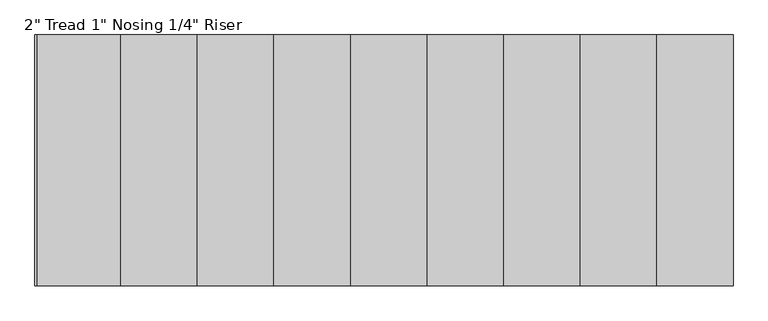
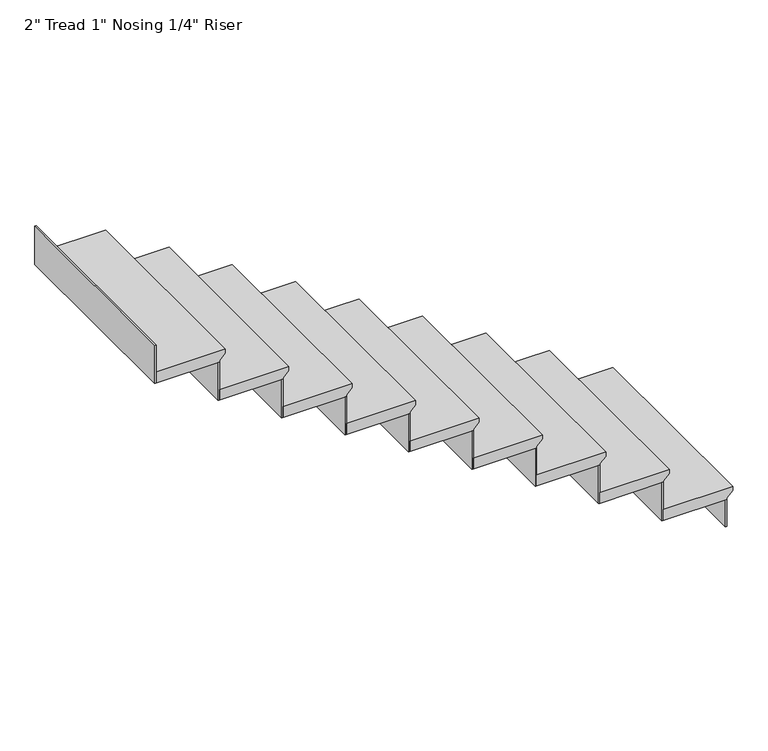
"""IFC4 building model written with IfcOpenShell, lengths in millimetres: stair flight geometry."""

from ifc_helpers import new_model, si_unit, origin, place, context, project, spatial, faceted_brep, source, transform, mapped, element, save


def stair_flight_6bca3b3f(model_context):
    return source(origin(), model_context, "Body", "Brep", [
        faceted_brep([(-9543.8120641, -2647.9669819, 3968.75), (-9543.8120641, -2647.9669819, 3987.8), (-9543.8120641, -3562.3669819, 3987.8), (-9543.8120641, -3562.3669819, 3968.75), (-9569.2120641, -2647.9669819, 3943.35), (-9569.2120641, -3562.3669819, 3943.35), (-9848.6120641, -2647.9669819, 3987.8), (-9848.6120641, -3562.3669819, 3987.8), (-9569.2120641, -3562.3669819, 3937.0), (-9848.6120641, -3562.3669819, 3937.0), (-9848.6120641, -2647.9669819, 3937.0), (-9569.2120641, -2647.9669819, 3937.0)], [[[0, 1, 2, 3]], [[4, 0, 3, 5]], [[2, 1, 6, 7]], [[8, 9, 10, 11]], [[2, 7, 9, 8, 5, 3]], [[8, 11, 4, 5]], [[6, 1, 0, 4, 11, 10]], [[7, 6, 10, 9]]]),
        faceted_brep([(-9569.2120641, -2647.9669819, 3937.0), (-9569.2120641, -2647.9669819, 3810.0), (-9575.5620641, -2647.9669819, 3810.0), (-9575.5620641, -2647.9669819, 3937.0), (-9569.2120641, -3562.3669819, 3937.0), (-9575.5620641, -3562.3669819, 3937.0), (-9575.5620641, -3562.3669819, 3810.0), (-9569.2120641, -3562.3669819, 3810.0)], [[[0, 1, 2, 3]], [[4, 5, 6, 7]], [[1, 0, 4, 7]], [[2, 1, 7, 6]], [[3, 2, 6, 5]], [[0, 3, 5, 4]]]),
        faceted_brep([(-9848.6120641, -2647.9669819, 4114.8), (-9848.6120641, -2647.9669819, 3937.0), (-9854.9620641, -2647.9669819, 3937.0), (-9854.9620641, -2647.9669819, 4114.8), (-9848.6120641, -3562.3669819, 4114.8), (-9854.9620641, -3562.3669819, 4114.8), (-9854.9620641, -3562.3669819, 3937.0), (-9848.6120641, -3562.3669819, 3937.0)], [[[0, 1, 2, 3]], [[4, 5, 6, 7]], [[1, 0, 4, 7]], [[2, 1, 7, 6]], [[3, 2, 6, 5]], [[0, 3, 5, 4]]]),
        faceted_brep([(-9823.2120641, -3562.3669819, 4165.6), (-9823.2120641, -2647.9669819, 4165.6), (-10128.0120641, -2647.9669819, 4165.6), (-10128.0120641, -3562.3669819, 4165.6), (-9848.6120641, -3562.3669819, 4114.8), (-10128.0120641, -3562.3669819, 4114.8), (-10128.0120641, -2647.9669819, 4114.8), (-9848.6120641, -2647.9669819, 4114.8), (-9848.6120641, -3562.3669819, 4121.15), (-9823.2120641, -3562.3669819, 4146.55), (-9848.6120641, -2647.9669819, 4121.15), (-9823.2120641, -2647.9669819, 4146.55)], [[[0, 1, 2, 3]], [[4, 5, 6, 7]], [[0, 3, 5, 4, 8, 9]], [[4, 7, 10, 8]], [[2, 1, 11, 10, 7, 6]], [[3, 2, 6, 5]], [[11, 1, 0, 9]], [[10, 11, 9, 8]]]),
        faceted_brep([(-10128.0120641, -2647.9669819, 4292.6), (-10128.0120641, -2647.9669819, 4114.8), (-10134.3620641, -2647.9669819, 4114.8), (-10134.3620641, -2647.9669819, 4292.6), (-10128.0120641, -3562.3669819, 4292.6), (-10134.3620641, -3562.3669819, 4292.6), (-10134.3620641, -3562.3669819, 4114.8), (-10128.0120641, -3562.3669819, 4114.8)], [[[0, 1, 2, 3]], [[4, 5, 6, 7]], [[1, 0, 4, 7]], [[2, 1, 7, 6]], [[3, 2, 6, 5]], [[0, 3, 5, 4]]]),
        faceted_brep([(-10102.6120641, -3562.3669819, 4343.4), (-10102.6120641, -2647.9669819, 4343.4), (-10407.4120641, -2647.9669819, 4343.4), (-10407.4120641, -3562.3669819, 4343.4), (-10128.0120641, -3562.3669819, 4292.6), (-10407.4120641, -3562.3669819, 4292.6), (-10407.4120641, -2647.9669819, 4292.6), (-10128.0120641, -2647.9669819, 4292.6), (-10128.0120641, -3562.3669819, 4298.95), (-10102.6120641, -3562.3669819, 4324.35), (-10128.0120641, -2647.9669819, 4298.95), (-10102.6120641, -2647.9669819, 4324.35)], [[[0, 1, 2, 3]], [[4, 5, 6, 7]], [[0, 3, 5, 4, 8, 9]], [[4, 7, 10, 8]], [[2, 1, 11, 10, 7, 6]], [[3, 2, 6, 5]], [[11, 1, 0, 9]], [[10, 11, 9, 8]]]),
        faceted_brep([(-10407.4120641, -2647.9669819, 4470.4), (-10407.4120641, -2647.9669819, 4292.6), (-10413.7620641, -2647.9669819, 4292.6), (-10413.7620641, -2647.9669819, 4470.4), (-10407.4120641, -3562.3669819, 4470.4), (-10413.7620641, -3562.3669819, 4470.4), (-10413.7620641, -3562.3669819, 4292.6), (-10407.4120641, -3562.3669819, 4292.6)], [[[0, 1, 2, 3]], [[4, 5, 6, 7]], [[1, 0, 4, 7]], [[2, 1, 7, 6]], [[3, 2, 6, 5]], [[0, 3, 5, 4]]]),
        faceted_brep([(-10382.0120641, -3562.3669819, 4521.2), (-10382.0120641, -2647.9669819, 4521.2), (-10686.8120641, -2647.9669819, 4521.2), (-10686.8120641, -3562.3669819, 4521.2), (-10407.4120641, -3562.3669819, 4470.4), (-10686.8120641, -3562.3669819, 4470.4), (-10686.8120641, -2647.9669819, 4470.4), (-10407.4120641, -2647.9669819, 4470.4), (-10407.4120641, -3562.3669819, 4476.75), (-10382.0120641, -3562.3669819, 4502.15), (-10407.4120641, -2647.9669819, 4476.75), (-10382.0120641, -2647.9669819, 4502.15)], [[[0, 1, 2, 3]], [[4, 5, 6, 7]], [[0, 3, 5, 4, 8, 9]], [[4, 7, 10, 8]], [[2, 1, 11, 10, 7, 6]], [[3, 2, 6, 5]], [[11, 1, 0, 9]], [[10, 11, 9, 8]]]),
        faceted_brep([(-10686.8120641, -2647.9669819, 4648.2), (-10686.8120641, -2647.9669819, 4470.4), (-10693.1620641, -2647.9669819, 4470.4), (-10693.1620641, -2647.9669819, 4648.2), (-10686.8120641, -3562.3669819, 4648.2), (-10693.1620641, -3562.3669819, 4648.2), (-10693.1620641, -3562.3669819, 4470.4), (-10686.8120641, -3562.3669819, 4470.4)], [[[0, 1, 2, 3]], [[4, 5, 6, 7]], [[1, 0, 4, 7]], [[2, 1, 7, 6]], [[3, 2, 6, 5]], [[0, 3, 5, 4]]]),
        faceted_brep([(-10661.4120641, -3562.3669819, 4699.0), (-10661.4120641, -2647.9669819, 4699.0), (-10966.2120641, -2647.9669819, 4699.0), (-10966.2120641, -3562.3669819, 4699.0), (-10686.8120641, -3562.3669819, 4648.2), (-10966.2120641, -3562.3669819, 4648.2), (-10966.2120641, -2647.9669819, 4648.2), (-10686.8120641, -2647.9669819, 4648.2), (-10686.8120641, -3562.3669819, 4654.55), (-10661.4120641, -3562.3669819, 4679.95), (-10686.8120641, -2647.9669819, 4654.55), (-10661.4120641, -2647.9669819, 4679.95)], [[[0, 1, 2, 3]], [[4, 5, 6, 7]], [[0, 3, 5, 4, 8, 9]], [[4, 7, 10, 8]], [[2, 1, 11, 10, 7, 6]], [[3, 2, 6, 5]], [[11, 1, 0, 9]], [[10, 11, 9, 8]]]),
        faceted_brep([(-10966.2120641, -2647.9669819, 4826.0), (-10966.2120641, -2647.9669819, 4648.2), (-10972.5620641, -2647.9669819, 4648.2), (-10972.5620641, -2647.9669819, 4826.0), (-10966.2120641, -3562.3669819, 4826.0), (-10972.5620641, -3562.3669819, 4826.0), (-10972.5620641, -3562.3669819, 4648.2), (-10966.2120641, -3562.3669819, 4648.2)], [[[0, 1, 2, 3]], [[4, 5, 6, 7]], [[1, 0, 4, 7]], [[2, 1, 7, 6]], [[3, 2, 6, 5]], [[0, 3, 5, 4]]]),
        faceted_brep([(-10940.8120641, -3562.3669819, 4876.8), (-10940.8120641, -2647.9669819, 4876.8), (-11245.6120641, -2647.9669819, 4876.8), (-11245.6120641, -3562.3669819, 4876.8), (-10966.2120641, -3562.3669819, 4826.0), (-11245.6120641, -3562.3669819, 4826.0), (-11245.6120641, -2647.9669819, 4826.0), (-10966.2120641, -2647.9669819, 4826.0), (-10966.2120641, -3562.3669819, 4832.35), (-10940.8120641, -3562.3669819, 4857.75), (-10966.2120641, -2647.9669819, 4832.35), (-10940.8120641, -2647.9669819, 4857.75)], [[[0, 1, 2, 3]], [[4, 5, 6, 7]], [[0, 3, 5, 4, 8, 9]], [[4, 7, 10, 8]], [[2, 1, 11, 10, 7, 6]], [[3, 2, 6, 5]], [[11, 1, 0, 9]], [[10, 11, 9, 8]]]),
        faceted_brep([(-11245.6120641, -2647.9669819, 5003.8), (-11245.6120641, -2647.9669819, 4826.0), (-11251.9620641, -2647.9669819, 4826.0), (-11251.9620641, -2647.9669819, 5003.8), (-11245.6120641, -3562.3669819, 5003.8), (-11251.9620641, -3562.3669819, 5003.8), (-11251.9620641, -3562.3669819, 4826.0), (-11245.6120641, -3562.3669819, 4826.0)], [[[0, 1, 2, 3]], [[4, 5, 6, 7]], [[1, 0, 4, 7]], [[2, 1, 7, 6]], [[3, 2, 6, 5]], [[0, 3, 5, 4]]]),
        faceted_brep([(-11220.2120641, -3562.3669819, 5054.6), (-11220.2120641, -2647.9669819, 5054.6), (-11525.0120641, -2647.9669819, 5054.6), (-11525.0120641, -3562.3669819, 5054.6), (-11245.6120641, -3562.3669819, 5003.8), (-11525.0120641, -3562.3669819, 5003.8), (-11525.0120641, -2647.9669819, 5003.8), (-11245.6120641, -2647.9669819, 5003.8), (-11245.6120641, -3562.3669819, 5010.15), (-11220.2120641, -3562.3669819, 5035.55), (-11245.6120641, -2647.9669819, 5010.15), (-11220.2120641, -2647.9669819, 5035.55)], [[[0, 1, 2, 3]], [[4, 5, 6, 7]], [[0, 3, 5, 4, 8, 9]], [[4, 7, 10, 8]], [[2, 1, 11, 10, 7, 6]], [[3, 2, 6, 5]], [[11, 1, 0, 9]], [[10, 11, 9, 8]]]),
        faceted_brep([(-11525.0120641, -2647.9669819, 5181.6), (-11525.0120641, -2647.9669819, 5003.8), (-11531.3620641, -2647.9669819, 5003.8), (-11531.3620641, -2647.9669819, 5181.6), (-11525.0120641, -3562.3669819, 5181.6), (-11531.3620641, -3562.3669819, 5181.6), (-11531.3620641, -3562.3669819, 5003.8), (-11525.0120641, -3562.3669819, 5003.8)], [[[0, 1, 2, 3]], [[4, 5, 6, 7]], [[1, 0, 4, 7]], [[2, 1, 7, 6]], [[3, 2, 6, 5]], [[0, 3, 5, 4]]]),
        faceted_brep([(-11499.6120641, -3562.3669819, 5232.4), (-11499.6120641, -2647.9669819, 5232.4), (-11804.4120641, -2647.9669819, 5232.4), (-11804.4120641, -3562.3669819, 5232.4), (-11525.0120641, -3562.3669819, 5181.6), (-11804.4120641, -3562.3669819, 5181.6), (-11804.4120641, -2647.9669819, 5181.6), (-11525.0120641, -2647.9669819, 5181.6), (-11525.0120641, -3562.3669819, 5187.95), (-11499.6120641, -3562.3669819, 5213.35), (-11525.0120641, -2647.9669819, 5187.95), (-11499.6120641, -2647.9669819, 5213.35)], [[[0, 1, 2, 3]], [[4, 5, 6, 7]], [[0, 3, 5, 4, 8, 9]], [[4, 7, 10, 8]], [[2, 1, 11, 10, 7, 6]], [[3, 2, 6, 5]], [[11, 1, 0, 9]], [[10, 11, 9, 8]]]),
        faceted_brep([(-12083.8120641, -2647.9669819, 5537.2), (-12083.8120641, -2647.9669819, 5359.4), (-12090.1620641, -2647.9669819, 5359.4), (-12090.1620641, -2647.9669819, 5537.2), (-12083.8120641, -3562.3669819, 5537.2), (-12090.1620641, -3562.3669819, 5537.2), (-12090.1620641, -3562.3669819, 5359.4), (-12083.8120641, -3562.3669819, 5359.4)], [[[0, 1, 2, 3]], [[4, 5, 6, 7]], [[1, 0, 4, 7]], [[2, 1, 7, 6]], [[3, 2, 6, 5]], [[0, 3, 5, 4]]]),
        faceted_brep([(-11804.4120641, -2647.9669819, 5359.4), (-11804.4120641, -2647.9669819, 5181.6), (-11810.7620641, -2647.9669819, 5181.6), (-11810.7620641, -2647.9669819, 5359.4), (-11804.4120641, -3562.3669819, 5359.4), (-11810.7620641, -3562.3669819, 5359.4), (-11810.7620641, -3562.3669819, 5181.6), (-11804.4120641, -3562.3669819, 5181.6)], [[[0, 1, 2, 3]], [[4, 5, 6, 7]], [[1, 0, 4, 7]], [[2, 1, 7, 6]], [[3, 2, 6, 5]], [[0, 3, 5, 4]]]),
        faceted_brep([(-11779.0120641, -3562.3669819, 5410.2), (-11779.0120641, -2647.9669819, 5410.2), (-12058.4120641, -2647.9669819, 5410.2), (-12083.8120641, -2647.9669819, 5410.2), (-12083.8120641, -3562.3669819, 5410.2), (-11804.4120641, -3562.3669819, 5359.4), (-12083.8120641, -3562.3669819, 5359.4), (-12083.8120641, -2647.9669819, 5359.4), (-12058.4120641, -2647.9669819, 5359.4), (-11804.4120641, -2647.9669819, 5359.4), (-11804.4120641, -3562.3669819, 5365.75), (-11779.0120641, -3562.3669819, 5391.15), (-11804.4120641, -2647.9669819, 5365.75), (-11779.0120641, -2647.9669819, 5391.15)], [[[0, 1, 2, 3, 4]], [[5, 6, 7, 8, 9]], [[0, 4, 6, 5, 10, 11]], [[5, 9, 12, 10]], [[2, 1, 13, 12, 9, 8]], [[3, 2, 8, 7]], [[4, 3, 7, 6]], [[13, 1, 0, 11]], [[12, 13, 11, 10]]]),
    ])


if __name__ == "__main__":
    model = new_model("IFC4")
    model_context = context("Model", 3, world=origin())
    ifc_project = project(units=[si_unit("LENGTHUNIT", "METRE", prefix="MILLI")], contexts=[model_context])
    site = spatial("IfcSite", under=ifc_project)
    building = spatial("IfcBuilding", under=site)
    placement = place(None, origin())
    stair_flight_shape = stair_flight_6bca3b3f(model_context)
    element("IfcStairFlight", 1, ObjectType="2\" Tread 1\" Nosing 1/4\" Riser", at=placement, inside=building, context=model_context, shape_type="MappedRepresentation", body=[
        mapped(stair_flight_shape, transform((0.0, 0.0, 0.0), x_axis=(1.0, 0.0, 0.0), y_axis=(0.0, 1.0, 0.0), z_axis=(0.0, 0.0, 1.0))),
    ])
    save(model, "model.ifc")
